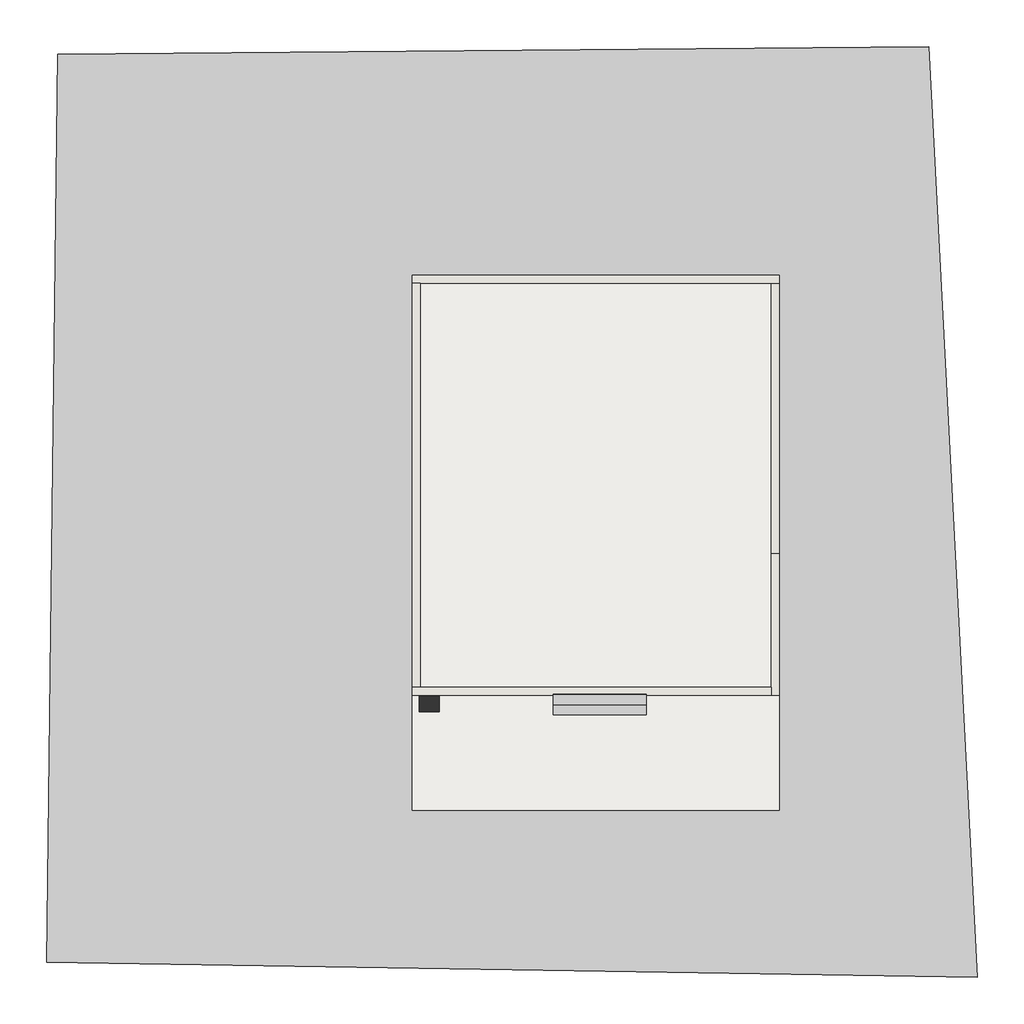
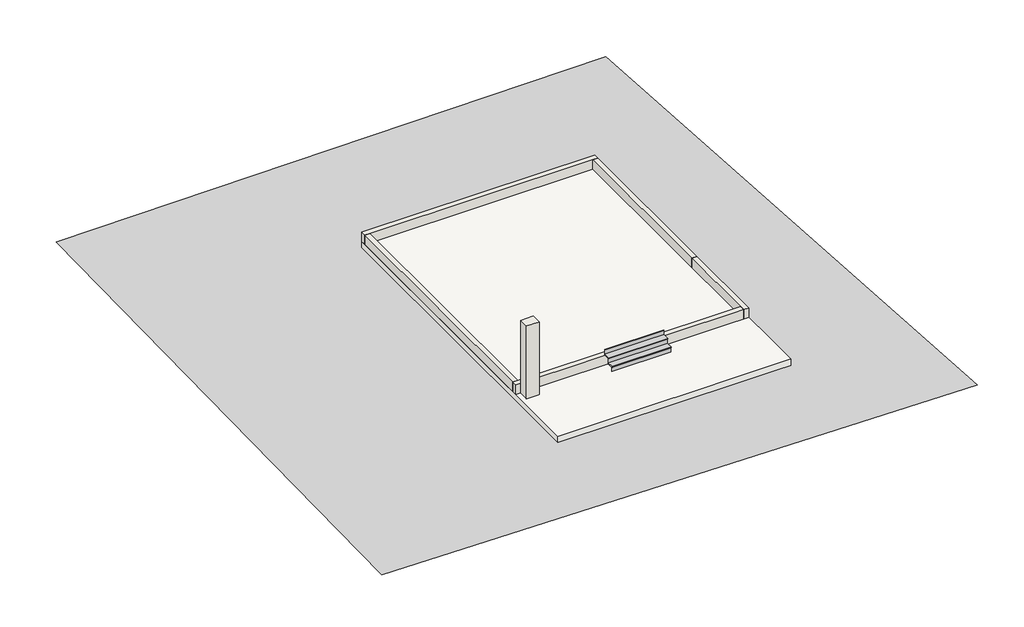
# One storey: 6 walls, 1 proxy, 1 slab, 1 stair flight.
"""IFC4 building model written with IfcOpenShell, lengths in millimetres."""

from ifc_helpers import new_model, si_unit, frame, origin, place, context, project, spatial, polyline, outline, extrude, faceted_brep, triangles, transform, mapped, element, save
from components import stair_flight_4a261924, walls_1_walls_1_84b2d317

model = new_model("IFC4")

# Units and contexts
model_context = context("Model", 3, world=origin())
ifc_project = project(units=[si_unit("LENGTHUNIT", "METRE", prefix="MILLI")], contexts=[model_context])

# Site, building, storey
site = spatial("IfcSite", under=ifc_project)
building = spatial("IfcBuilding", under=site)
storey = spatial("IfcBuildingStorey", under=building, Elevation=-762.0)

# Proxy
placement = place(None, origin())
element("IfcBuildingElementProxy", 1, Name="Building Element Proxy", at=placement, inside=storey, context=model_context, shape_type="Tessellation", body=[
    triangles([(-17085.0757507, 19459.1738617, -1066.8), (-17409.8501129, -6739.2595734, -1066.8), (9438.1314651, -7172.2918625, -1066.8), (8030.7778336, 19675.6897156, -1066.8)], [[1, 2, 4], [3, 4, 2]], closed=False),
])

# Slab
element("IfcSlab", 2, ObjectType="Generic - 12\"", at=placement, inside=storey, context=model_context, shape_type="SweptSolid", body=[
    extrude(outline(polyline([(3726.6918749, 13083.8953049), (3726.6918749, -2346.6046951), (-6865.1081251, -2346.6046951), (-6865.1081251, 13083.8953049), (3726.6918749, 13083.8953049)])), frame((0.0, 0.0, -1066.8), z_axis=(0.0, 0.0, 1.0), x_axis=(1.0, 0.0, 0.0)), (0.0, 0.0, 1.0), 304.8),
])

# Stair flight
stair_flight_shape = stair_flight_4a261924(model_context)
element("IfcStairFlight", 3, ObjectType="2\" Tread 1\" Nosing 1/4\" Riser", at=placement, inside=storey, context=model_context, shape_type="MappedRepresentation", body=[
    mapped(stair_flight_shape, transform((0.0, 0.0, 0.0), x_axis=(1.0, 0.0, 0.0), y_axis=(0.0, 1.0, 0.0), z_axis=(0.0, 0.0, 1.0))),
])

# Walls
element("IfcWall", 4, ObjectType="9\"", at=placement, inside=storey, context=model_context, shape_type="Brep", body=[
    faceted_brep([(-6865.1081251, 12855.2953049, -762.0), (-6636.5081251, 12855.2953049, -762.0), (3498.0918749, 12855.2953049, -762.0), (3726.6918749, 12855.2953049, -762.0), (3726.6918749, 12855.2953049, -304.8), (3498.0918749, 12855.2953049, -304.8), (-6636.5081251, 12855.2953049, -304.8), (-6865.1081251, 12855.2953049, -304.8), (-6865.1081251, 13083.8953049, -762.0), (-6865.1081251, 13083.8953049, -304.8), (3726.6918749, 13083.8953049, -304.8), (3726.6918749, 13083.8953049, -762.0)], [[[0, 1, 2, 3, 4, 5, 6, 7]], [[8, 9, 10, 11]], [[3, 2, 1, 0, 8, 11]], [[7, 6, 5, 4, 10, 9]], [[4, 3, 11, 10]], [[0, 7, 9, 8]]]),
])
element("IfcWall", 5, ObjectType="9\"", at=placement, inside=storey, context=model_context, shape_type="SweptSolid", body=[
    extrude(outline(polyline([(3498.0918749, 5044.7953049), (3498.0918749, 12855.2953049), (3726.6918749, 12855.2953049), (3726.6918749, 5044.7953049), (3498.0918749, 5044.7953049)])), frame((0.0, 0.0, -762.0), z_axis=(0.0, 0.0, 1.0), x_axis=(1.0, 0.0, 0.0)), (0.0, 0.0, 1.0), 457.2),
])
element("IfcWall", 6, ObjectType="9\"", at=placement, inside=storey, context=model_context, shape_type="Brep", body=[
    faceted_brep([(3498.0918749, 1196.6953049, -762.0), (-6636.5081251, 1196.6953049, -762.0), (-6865.1081251, 1196.6953049, -762.0), (-6865.1081251, 1196.6953049, -304.8), (-6636.5081251, 1196.6953049, -304.8), (3498.0918749, 1196.6953049, -304.8), (3498.0918749, 968.0953049, -762.0), (3498.0918749, 968.0953049, -304.8), (-6865.1081251, 968.0953049, -304.8), (-6865.1081251, 968.0953049, -762.0)], [[[0, 1, 2, 3, 4, 5]], [[6, 7, 8, 9]], [[2, 1, 0, 6, 9]], [[5, 4, 3, 8, 7]], [[3, 2, 9, 8]], [[0, 5, 7, 6]]]),
])
element("IfcWall", 7, ObjectType="9\"", at=placement, inside=storey, context=model_context, shape_type="SweptSolid", body=[
    extrude(outline(polyline([(-6636.5081251, 12855.2953049), (-6636.5081251, 1196.6953049), (-6865.1081251, 1196.6953049), (-6865.1081251, 12855.2953049), (-6636.5081251, 12855.2953049)])), frame((0.0, 0.0, -762.0), z_axis=(0.0, 0.0, 1.0), x_axis=(1.0, 0.0, 0.0)), (0.0, 0.0, 1.0), 457.2),
])
element("IfcWall", 8, ObjectType="9\"", at=placement, inside=storey, context=model_context, shape_type="Brep", body=[
    faceted_brep([(3498.0918749, 968.0953049, -304.8), (3498.0918749, 1196.6953049, -304.8), (3498.0918749, 5044.7953049, -304.8), (3498.0918749, 5044.7953049, -762.0), (3498.0918749, 1196.6953049, -762.0), (3498.0918749, 968.0953049, -762.0), (3726.6918749, 968.0953049, -304.8), (3726.6918749, 968.0953049, -762.0), (3726.6918749, 5044.7953049, -762.0), (3726.6918749, 5044.7953049, -304.8)], [[[0, 1, 2, 3, 4, 5]], [[6, 7, 8, 9]], [[2, 1, 0, 6, 9]], [[5, 4, 3, 8, 7]], [[3, 2, 9, 8]], [[0, 5, 7, 6]]]),
])
walls_1_walls_1_shape = walls_1_walls_1_84b2d317(model_context)
element("IfcWall", 9, ObjectType="Walls 1 : Walls 1", at=placement, inside=storey, context=model_context, shape_type="MappedRepresentation", body=[
    mapped(walls_1_walls_1_shape, transform((0.0, 0.0, 0.0), x_axis=(1.0, 0.0, 0.0), y_axis=(0.0, 1.0, 0.0), z_axis=(0.0, 0.0, 1.0))),
])

save(model, "model.ifc")

# Revit data of these elements
# Type "Generic - 12\""
#   Assembly Code = "B1010"
#   Function = 0
#   Layers, outside or top first: 1' - 0" no material (function 1)
# Type "9\""
#   Assembly Code = "B2010"
#   Layers, outside or top first: 0' - 9" "1 wall" (function 1)
# Element 1 (IfcBuildingElementProxy)
#   Material = none
#   Phase Created = New Construction
# Element 2 (IfcSlab, "Generic - 12\"")
#   Height Offset From Level = 0' - 0"
#   Phase Created = New Construction
#   Materials on its faces: "Default Floor", "1 white"
# Element 3 (IfcStairFlight, "2\" Tread 1\" Nosing 1/4\" Riser")
#   Phase Created = New Construction
#   Materials on its faces: "1 white"
# Elements 4, 5, 6, 7, 8 (IfcWall, "9\"")
#   Top Offset = 0' - 0"
#   Base Offset = 0' - 0"
#   Unconnected Height = 1' - 6"
#   wall height = 1' - 6"
#   Phase Created = New Construction
#   Materials on its faces: "1 wall"
# Element 9 (IfcWall, "Walls 1 : Walls 1")
#   Phase Created = New Construction
#   Materials on its faces: "1 white", "Default Wall"
# Materials
#   "1 wall": class "Generic", colour RGB 172 157 136, transparency 0, Cost = 0
#   "Default Floor": colour RGB 128 128 128, transparency 0, Cost = 0
#   "1 white": class "Generic", colour RGB 244 245 241, transparency 0, Cost = 0
#   "Default Wall": colour RGB 128 128 128, transparency 0, Cost = 0
